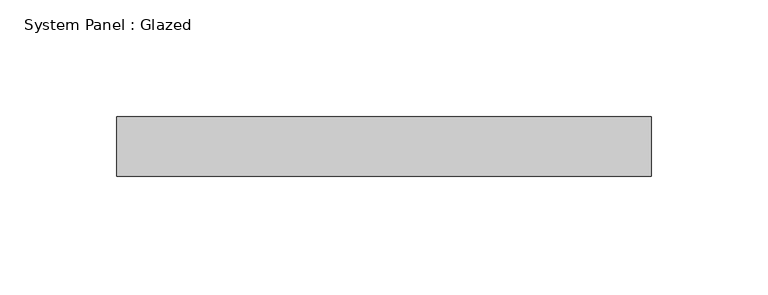
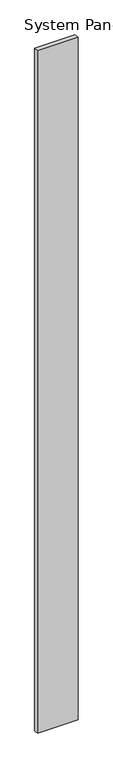
"""IFC4 building model written with IfcOpenShell, lengths in millimetres: plate geometry, System Panel : Glazed."""

from ifc_helpers import new_model, si_unit, origin, origin_with_axes, place, context, project, spatial, polyline, outline, extrude, source, transform, mapped, element, save


def system_panel_glazed_5b01c733(model_context):
    return source(origin(), model_context, "Body", "SweptSolid", [
        extrude(outline(polyline([(114.3, 19.05), (-114.3, 19.05), (-114.3, 44.45), (114.3, 44.45), (114.3, 19.05)])), origin_with_axes(), (0.0, 0.0, 1.0), 4062.3470043),
    ])


if __name__ == "__main__":
    model = new_model("IFC4")
    model_context = context("Model", 3, world=origin())
    ifc_project = project(units=[si_unit("LENGTHUNIT", "METRE", prefix="MILLI")], contexts=[model_context])
    site = spatial("IfcSite", under=ifc_project)
    building = spatial("IfcBuilding", under=site)
    placement = place(None, origin())
    system_panel_glazed_shape = system_panel_glazed_5b01c733(model_context)
    element("IfcPlate", 1, ObjectType="System Panel : Glazed", at=placement, inside=building, context=model_context, shape_type="MappedRepresentation", body=[
        mapped(system_panel_glazed_shape, transform((0.0, 0.0, 0.0), x_axis=(1.0, 0.0, 0.0), y_axis=(0.0, 1.0, 0.0), z_axis=(0.0, 0.0, 1.0))),
    ])
    save(model, "model.ifc")

# Revit data of these elements
# Type "System Panel : Glazed"
#   Construction Type Id = "GSP4R"
#   Analytic Construction = "1/8 in Pilkington single glazing"
#   Visual Light Transmittance = 0.9
#   Solar Heat Gain Coefficient = 0.86
#   Heat Transfer Coefficient (U) = 1.18115 BTU/(h·ft²·°F)
#   Define Thermal Properties by = 1
# Element 1 (IfcPlate, "System Panel : Glazed")
#   Materials on its faces: "Glass"
# Materials
#   "Glass": class "Glass", colour RGB 0 128 192, transparency 0.75, Description = "Soda Lime Glass", Cost = 0
